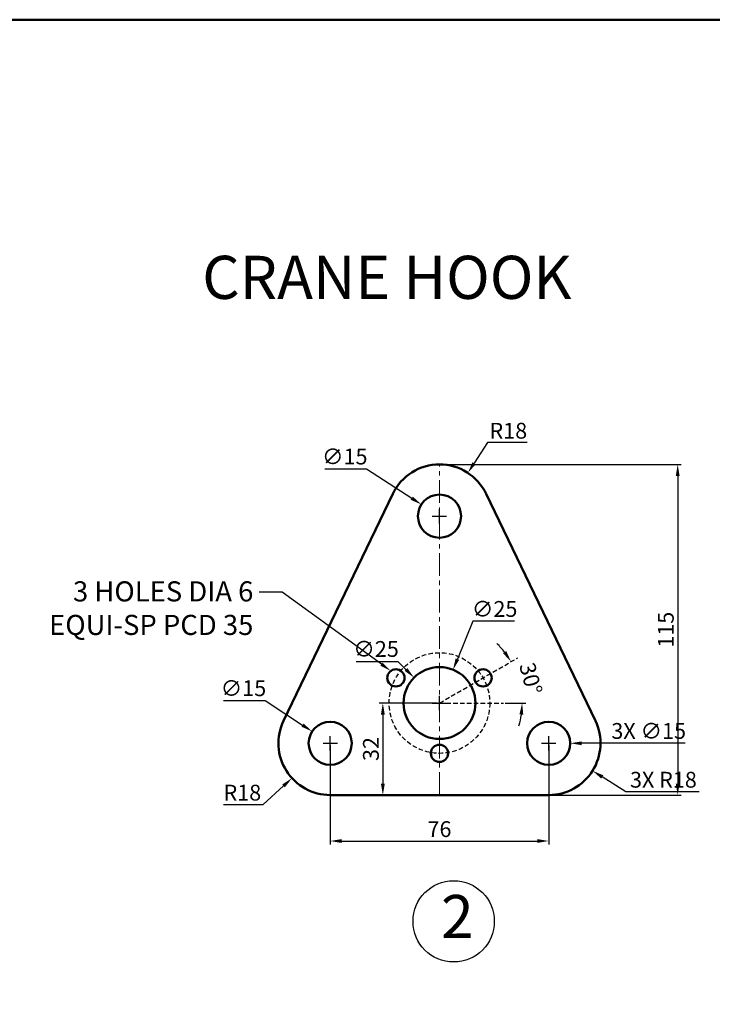
# Model space of a CAD drawing. Units: millimetres. Extents: x -3 to 930, y -425 to 322.
# Tile 4 of 5: x 288 to 529, y -21 to 322. Entities that reach past the tile are written whole.
import ezdxf
from ezdxf import colors
from ezdxf.entities.mleader import LeaderData, LeaderLine
from ezdxf.math import Vec2, Vec3

# ---------------------------------------------------------------- set-up
doc = ezdxf.new("R2010")
doc.units = ezdxf.units.MM
doc.header["$LTSCALE"] = 0.5
doc.linetypes.add('CENTER', pattern=[50.8, 31.75, -6.35, 6.35, -6.35])
doc.linetypes.add('HIDDEN', pattern=[9.525, 6.35, -3.175])
for name, color, linetype, lineweight in [('M-ANNO-SYMB', 3, 'Continuous', 25), ('M-CNTR', 1, 'CENTER', 18), ('M-DIMS', 2, 'Continuous', 25), ('M-HIDN', 4, 'HIDDEN', 25), ('M-OUTL', 7, 'Continuous', 50), ('M-TEXT', 3, 'Continuous', 25)]:
    doc.layers.add(name, color=color, linetype=linetype, lineweight=lineweight)
doc.styles.get("Standard").update_dxf_attribs({"font": 'arial.ttf'})
doc.dimstyles.new('ISO-25', dxfattribs={"dimtxt": 5.5, "dimasz": 4, "dimexe": 1.25, "dimexo": 0.625, "dimtad": 1, "dimtoh": 1, "dimdec": 0, "dimtxsty": 'Standard', "dimcen": 2.5, "dimadec": 0, "dimazin": 0, "dimtfac": 1, "dimtdec": 0, "dimtofl": 0, "dimtmove": 0, "dimatfit": 3, "dimfxl": 1, "dimarcsym": 0})

# ---------------------------------------------------------------- blocks, each defined once
blk = doc.blocks.new('*D19')
at = {"layer": 'Defpoints', "color": 0, "ltscale": 0.5, "transparency": 16777216}
for p in [(396.31, 69.97), (472.31, 69.97), (472.31, 35.98)]:
    blk.add_point(p, dxfattribs=at)
at = {"layer": 'M-DIMS', "color": 0, "lineweight": -2, "ltscale": 0.5, "transparency": 16777216}
for p, q in [((396.31, 69.35), (396.31, 34.73)), ((472.31, 69.35), (472.31, 34.73)), ((400.31, 35.98), (468.31, 35.98))]:
    blk.add_line(p, q, dxfattribs=at)
at = {"layer": 'M-DIMS', "color": 0, "ltscale": 0.5, "transparency": 16777216}
for points in [[(400.31, 36.65), (400.31, 35.31), (396.31, 35.98)], [(468.31, 36.65), (468.31, 35.31), (472.31, 35.98)]]:
    blk.add_solid(points, dxfattribs=at)
at = {"layer": 'M-DIMS', "color": 0, "ltscale": 0.5, "transparency": 16777216, "insert": (434.31, 39.41), "char_height": 5.5, "attachment_point": 5}
blk.add_mtext('76', dxfattribs=at)
blk = doc.blocks.new('*D20')
at = {"layer": 'Defpoints', "color": 0, "ltscale": 0.5, "transparency": 16777216}
for p in [(434.31, 166.97), (434.31, 51.97), (517.16, 51.97)]:
    blk.add_point(p, dxfattribs=at)
at = {"layer": 'M-DIMS', "color": 0, "lineweight": -2, "ltscale": 0.5, "transparency": 16777216}
for p, q in [((434.93, 166.97), (518.41, 166.97)), ((517.16, 162.97), (517.16, 55.97)), ((434.93, 51.97), (518.41, 51.97))]:
    blk.add_line(p, q, dxfattribs=at)
at = {"layer": 'M-DIMS', "color": 0, "ltscale": 0.5, "transparency": 16777216}
for points in [[(516.49, 162.97), (517.83, 162.97), (517.16, 166.97)], [(516.49, 55.97), (517.83, 55.97), (517.16, 51.97)]]:
    blk.add_solid(points, dxfattribs=at)
at = {"layer": 'M-DIMS', "color": 0, "ltscale": 0.5, "transparency": 16777216, "insert": (513.73, 109.47), "char_height": 5.5, "attachment_point": 5, "rotation": 90}
blk.add_mtext('115', dxfattribs=at)
blk = doc.blocks.new('*D21')
at = {"layer": 'Defpoints', "color": 0, "ltscale": 0.5, "transparency": 16777216}
for p in [(396.31, 69.97), (383.02, 57.84)]:
    blk.add_point(p, dxfattribs=at)
at = {"layer": 'M-DIMS', "color": 0, "lineweight": -2, "ltscale": 0.5, "transparency": 16777216}
for p, q in [((396.31, 67.47), (396.31, 72.47)), ((393.81, 69.97), (398.81, 69.97)), ((372.96, 48.65), (380.06, 55.14)), ((359.19, 48.65), (372.96, 48.65))]:
    blk.add_line(p, q, dxfattribs=at)
at = {"layer": 'M-DIMS', "color": 0, "ltscale": 0.5, "transparency": 16777216}
blk.add_solid([(379.62, 55.63), (380.51, 54.65), (383.02, 57.84)], dxfattribs=at)
at = {"layer": 'M-DIMS', "color": 0, "ltscale": 0.5, "transparency": 16777216, "insert": (365.76, 52.09), "char_height": 5.5, "attachment_point": 5}
blk.add_mtext('R18', dxfattribs=at)
blk = doc.blocks.new('*D22')
at = {"layer": 'Defpoints', "color": 0, "ltscale": 0.5, "transparency": 16777216}
for p in [(444.17, 164.03), (434.31, 148.97)]:
    blk.add_point(p, dxfattribs=at)
at = {"layer": 'M-DIMS', "color": 0, "lineweight": -2, "ltscale": 0.5, "transparency": 16777216}
for p, q in [((451.06, 174.55), (446.36, 167.38)), ((464.83, 174.55), (451.06, 174.55)), ((434.31, 146.47), (434.31, 151.47)), ((431.81, 148.97), (436.81, 148.97))]:
    blk.add_line(p, q, dxfattribs=at)
at = {"layer": 'M-DIMS', "color": 0, "ltscale": 0.5, "transparency": 16777216}
blk.add_solid([(445.8, 167.74), (446.92, 167.01), (444.17, 164.03)], dxfattribs=at)
at = {"layer": 'M-DIMS', "color": 0, "ltscale": 0.5, "transparency": 16777216, "insert": (458.26, 177.98), "char_height": 5.5, "attachment_point": 5}
blk.add_mtext('R18', dxfattribs=at)
blk = doc.blocks.new('*D23')
at = {"layer": 'Defpoints', "color": 0, "ltscale": 0.5, "transparency": 16777216}
for p in [(428.02, 153.05), (440.6, 144.89)]:
    blk.add_point(p, dxfattribs=at)
at = {"layer": 'M-DIMS', "color": 0, "lineweight": -2, "ltscale": 0.5, "transparency": 16777216}
for p, q in [((394.42, 165.41), (408.95, 165.41)), ((408.95, 165.41), (424.66, 155.23)), ((434.31, 146.47), (434.31, 151.47)), ((431.81, 148.97), (436.81, 148.97))]:
    blk.add_line(p, q, dxfattribs=at)
at = {"layer": 'M-DIMS', "color": 0, "ltscale": 0.5, "transparency": 16777216}
blk.add_solid([(425.02, 155.79), (424.3, 154.67), (428.02, 153.05)], dxfattribs=at)
at = {"layer": 'M-DIMS', "color": 0, "ltscale": 0.5, "transparency": 16777216, "insert": (401.37, 169), "char_height": 5.5, "attachment_point": 5}
blk.add_mtext('∅15', dxfattribs=at)
blk = doc.blocks.new('*D24')
at = {"layer": 'Defpoints', "color": 0, "ltscale": 0.5, "transparency": 16777216}
for p in [(390.04, 74.09), (402.58, 65.86)]:
    blk.add_point(p, dxfattribs=at)
at = {"layer": 'M-DIMS', "color": 0, "lineweight": -2, "ltscale": 0.5, "transparency": 16777216}
for p, q in [((359.18, 84.82), (373.7, 84.82)), ((373.7, 84.82), (386.7, 76.29)), ((396.31, 67.47), (396.31, 72.47)), ((393.81, 69.97), (398.81, 69.97))]:
    blk.add_line(p, q, dxfattribs=at)
at = {"layer": 'M-DIMS', "color": 0, "ltscale": 0.5, "transparency": 16777216}
blk.add_solid([(387.06, 76.84), (386.33, 75.73), (390.04, 74.09)], dxfattribs=at)
at = {"layer": 'M-DIMS', "color": 0, "ltscale": 0.5, "transparency": 16777216, "insert": (366.13, 88.41), "char_height": 5.5, "attachment_point": 5}
blk.add_mtext('∅15', dxfattribs=at)
blk = doc.blocks.new('*D25')
at = {"layer": 'Defpoints', "color": 0, "ltscale": 0.5, "transparency": 16777216}
for p in [(439.03, 95.55), (429.59, 72.4)]:
    blk.add_point(p, dxfattribs=at)
at = {"layer": 'M-DIMS', "color": 0, "lineweight": -2, "ltscale": 0.5, "transparency": 16777216}
for p, q in [((445.92, 112.41), (440.55, 99.25)), ((460.45, 112.41), (445.92, 112.41)), ((434.31, 81.47), (434.31, 86.47)), ((431.81, 83.97), (436.81, 83.97))]:
    blk.add_line(p, q, dxfattribs=at)
at = {"layer": 'M-DIMS', "color": 0, "ltscale": 0.5, "transparency": 16777216}
blk.add_solid([(439.93, 99.5), (441.16, 99), (439.03, 95.55)], dxfattribs=at)
at = {"layer": 'M-DIMS', "color": 0, "ltscale": 0.5, "transparency": 16777216, "insert": (453.49, 115.99), "char_height": 5.5, "attachment_point": 5}
blk.add_mtext('∅25', dxfattribs=at)
blk = doc.blocks.new('*D26')
at = {"layer": 'Defpoints', "color": 0, "ltscale": 0.5, "transparency": 16777216}
for p in [(461.61, 99.74), (462.63, 88.97), (434.31, 83.97), (434.31, 83.97), (456.56, 83.97)]:
    blk.add_point(p, dxfattribs=at)
at = {"layer": 'M-DIMS', "color": 0, "lineweight": -2, "ltscale": 0.5, "transparency": 16777216}
blk.add_line((457.19, 83.97), (464.32, 83.97), dxfattribs=at)
for start, end in [(37.9764, 45.9529), (344.0471, 352.0236)]:
    blk.add_arc((434.31, 83.97), 28.76, start, end, dxfattribs=at)
at = {"layer": 'M-DIMS', "color": 0, "ltscale": 0.5, "transparency": 16777216}
for points in [[(457.53, 102.04), (456.42, 101.3), (459.21, 98.35)], [(462.12, 80.03), (463.45, 79.94), (463.07, 83.97)]]:
    blk.add_solid(points, dxfattribs=at)
at = {"layer": 'M-DIMS', "color": 0, "ltscale": 0.5, "transparency": 16777216, "insert": (465.4, 92.3), "char_height": 5.5, "attachment_point": 5, "rotation": 285}
blk.add_mtext('30°', dxfattribs=at)
blk = doc.blocks.new('*D27')
at = {"layer": 'Defpoints', "color": 0, "ltscale": 0.5, "transparency": 16777216}
for p in [(434.31, 83.97), (414.62, 51.97), (434.31, 51.97)]:
    blk.add_point(p, dxfattribs=at)
at = {"layer": 'M-DIMS', "color": 0, "lineweight": -2, "ltscale": 0.5, "transparency": 16777216}
for p, q in [((433.68, 83.97), (413.37, 83.97)), ((414.62, 79.97), (414.62, 55.97)), ((433.68, 51.97), (413.37, 51.97))]:
    blk.add_line(p, q, dxfattribs=at)
at = {"layer": 'M-DIMS', "color": 0, "ltscale": 0.5, "transparency": 16777216}
for points in [[(413.95, 79.97), (415.29, 79.97), (414.62, 83.97)], [(413.95, 55.97), (415.29, 55.97), (414.62, 51.97)]]:
    blk.add_solid(points, dxfattribs=at)
at = {"layer": 'M-DIMS', "color": 0, "ltscale": 0.5, "transparency": 16777216, "insert": (411.18, 67.97), "char_height": 5.5, "attachment_point": 5, "rotation": 90}
blk.add_mtext('32', dxfattribs=at)
blk = doc.blocks.new('BALLOON')
at = {"ltscale": 0.5}
blk.add_circle((198.15, 8.03), 14.13, dxfattribs=at)
blk = doc.blocks.new('*D92')
at = {"layer": 'Defpoints', "color": 0, "ltscale": 0.5, "transparency": 16777216}
for p in [(472.31, 69.97), (487.55, 60.39)]:
    blk.add_point(p, dxfattribs=at)
at = {"layer": 'M-DIMS', "color": 0, "lineweight": -2, "ltscale": 0.5, "transparency": 16777216}
for p, q in [((472.31, 67.47), (472.31, 72.47)), ((469.81, 69.97), (474.81, 69.97)), ((499.08, 53.14), (490.94, 58.26)), ((524.67, 53.14), (499.08, 53.14))]:
    blk.add_line(p, q, dxfattribs=at)
at = {"layer": 'M-DIMS', "color": 0, "ltscale": 0.5, "transparency": 16777216}
blk.add_solid([(491.29, 58.83), (490.58, 57.7), (487.55, 60.39)], dxfattribs=at)
at = {"layer": 'M-DIMS', "color": 0, "ltscale": 0.5, "transparency": 16777216, "insert": (512.19, 56.58), "char_height": 5.5, "attachment_point": 5}
blk.add_mtext('3X R18', dxfattribs=at)
blk = doc.blocks.new('*D93')
at = {"layer": 'Defpoints', "color": 0, "ltscale": 0.5, "transparency": 16777216}
for p in [(464.81, 69.98), (479.81, 69.97)]:
    blk.add_point(p, dxfattribs=at)
at = {"layer": 'M-DIMS', "color": 0, "lineweight": -2, "ltscale": 0.5, "transparency": 16777216}
for p, q in [((472.31, 67.47), (472.31, 72.47)), ((469.81, 69.97), (474.81, 69.97)), ((493.73, 69.96), (483.81, 69.97)), ((519.78, 69.96), (493.73, 69.96))]:
    blk.add_line(p, q, dxfattribs=at)
at = {"layer": 'M-DIMS', "color": 0, "ltscale": 0.5, "transparency": 16777216}
blk.add_solid([(483.81, 70.63), (483.81, 69.3), (479.81, 69.97)], dxfattribs=at)
at = {"layer": 'M-DIMS', "color": 0, "ltscale": 0.5, "transparency": 16777216, "insert": (507.07, 73.55), "char_height": 5.5, "attachment_point": 5}
blk.add_mtext('3X ∅15', dxfattribs=at)
blk = doc.blocks.new('*D94')
at = {"layer": 'Defpoints', "color": 0, "ltscale": 0.5, "transparency": 16777216}
for p in [(425.48, 92.82), (443.14, 75.13)]:
    blk.add_point(p, dxfattribs=at)
at = {"layer": 'M-DIMS', "color": 0, "lineweight": -2, "ltscale": 0.5, "transparency": 16777216}
for p, q in [((405.3, 98.48), (419.83, 98.48)), ((419.83, 98.48), (422.65, 95.65)), ((434.31, 81.47), (434.31, 86.47)), ((431.81, 83.97), (436.81, 83.97))]:
    blk.add_line(p, q, dxfattribs=at)
at = {"layer": 'M-DIMS', "color": 0, "ltscale": 0.5, "transparency": 16777216}
blk.add_solid([(423.13, 96.12), (422.18, 95.18), (425.48, 92.82)], dxfattribs=at)
at = {"layer": 'M-DIMS', "color": 0, "ltscale": 0.5, "transparency": 16777216, "insert": (412.25, 102.07), "char_height": 5.5, "attachment_point": 5}
blk.add_mtext('∅25', dxfattribs=at)

msp = doc.modelspace()

# ---------------------------------------------------------------- linework, layer by layer
at = {"layer": 'M-CNTR', "ltscale": 0.5}
msp.add_line((434.3099, 51.9733), (434.3099, 166.9733), dxfattribs=at)
at = {"layer": 'M-HIDN', "ltscale": 0.5}
for q in [(461.6109, 99.7356), (456.5633, 83.9733)]:
    msp.add_line((434.3099, 83.9733), q, dxfattribs=at)
msp.add_circle((434.3099, 83.9733), 17.5, dxfattribs=at)
at = {"layer": 'M-OUTL', "ltscale": 0.5}
for p, q in [((418.0889, 156.7759), (380.0889, 77.7759)), ((450.5309, 156.7759), (488.5309, 77.7759)), ((396.3099, 51.9733), (472.3099, 51.9733))]:
    msp.add_line(p, q, dxfattribs=at)
msp.add_lwpolyline([(-2.6134, 321.6785), (929.6113, 321.6785), (929.6113, -424.8872), (-2.6134, -424.8872)], close=True, dxfattribs=at)
for centre, radius in [((434.3099, 148.9733), 7.5), ((434.3099, 83.9733), 12.5), ((419.1545, 92.7233), 3), ((449.4654, 92.7233), 3), ((396.3099, 69.9733), 7.5), ((472.3099, 69.9733), 7.5), ((434.3099, 66.4733), 3)]:
    msp.add_circle(centre, radius, dxfattribs=at)
for centre, start, end in [((434.3099, 148.9733), 25.688143, 154.311857), ((396.3099, 69.9733), 154.311857, 270), ((472.3099, 69.9733), 270, 25.688143)]:
    msp.add_arc(centre, 18, start, end, dxfattribs=at)

# ---------------------------------------------------------------- block references
at = {"layer": 'M-ANNO-SYMB'}
msp.add_blockref('BALLOON', (241.1008, 0), dxfattribs=at)

# ---------------------------------------------------------------- texts
at = {"layer": 'M-TEXT', "ltscale": 0.5, "char_height": 15, "attachment_point": 1}
for s, width, insert in [('CRANE HOOK', 189.287448, (351.7987, 239.5512)), ('2', 15, (434.8526, 17.2084))]:
    msp.add_mtext_dynamic_manual_height_columns(s, width=width, gutter_width=12.5, heights=[0], dxfattribs=dict(at, insert=insert))

# ---------------------------------------------------------------- dimensions: what is measured, and where the dimension line sits
at = {"layer": 'M-DIMS', "ltscale": 0.5}
dim = msp.add_radius_dim(center=(434.3099, 148.9733), mpoint=(444.1699, 164.0326), dimstyle='ISO-25', override={"dimclrd": 0, "dimclre": 0, "dimclrt": 0}, dxfattribs=at)
dim.commit()
dim.dimension.update_dxf_attribs({"geometry": '*D22', "text_midpoint": (458.2571, 174.549), "dimtype": 164})
for p1, p2, override, picture, middle in [((440.6035, 144.894), (428.0164, 153.0527), {"dimclrd": 0, "dimclre": 0, "dimclrt": 0}, '*D23', (401.3735, 165.4108)), ((429.5856, 72.4005), (439.0342, 95.5462), {"dimclrd": 0, "dimclre": 0, "dimclrt": 0}, '*D25', (453.4933, 112.405)), ((443.1404, 75.1261), (425.4795, 92.8206), {"dimdec": 0, "dimlfac": 1, "dimrnd": 0, "dimzin": 0, "dimdsep": 46, "dimlunit": 2}, '*D94', (412.2511, 98.4828)), ((402.5787, 65.8561), (390.0411, 74.0906), {"dimclrd": 0, "dimclre": 0, "dimclrt": 0}, '*D24', (366.1273, 84.8206))]:
    dim = msp.add_diameter_dim_2p(p1=p1, p2=p2, dimstyle='ISO-25', override=override, dxfattribs=at)
    dim.commit()
    dim.dimension.update_dxf_attribs({"geometry": picture, "text_midpoint": middle, "dimtype": 163})
for base, p1, picture, middle in [((517.1601, 51.9733), (434.3099, 166.9733), '*D20', (513.7269, 109.4733)), ((414.6186, 51.9733), (434.3099, 83.9733), '*D27', (411.1836, 67.9733))]:
    dim = msp.add_linear_dim(base=base, p1=p1, p2=(434.3099, 51.9733), angle=90, dimstyle='ISO-25', override={"dimclrd": 0, "dimclre": 0, "dimclrt": 0}, dxfattribs=at)
    dim.commit()
    dim.dimension.update_dxf_attribs({"geometry": picture, "text_midpoint": middle})
dim = msp.add_angular_dim_2l(base=(462.6288, 88.9667), line1=((434.3099, 83.9733), (456.5633, 83.9733)), line2=((434.3099, 83.9733), (461.6109, 99.7356)), dimstyle='ISO-25', override={"dimclrd": 0, "dimclre": 0, "dimclrt": 0}, dxfattribs=at)
dim.commit()
dim.dimension.update_dxf_attribs({"geometry": '*D26', "text_midpoint": (465.4038, 92.3049)})
dim = msp.add_diameter_dim_2p(p1=(464.8099, 69.9767), p2=(479.8099, 69.97), text='3X <>', dimstyle='ISO-25', override={"dimdec": 0, "dimlfac": 1, "dimrnd": 0, "dimzin": 0, "dimdsep": 46, "dimlunit": 2}, dxfattribs=at)
dim.commit()
dim.dimension.update_dxf_attribs({"geometry": '*D93', "text_midpoint": (493.7339, 69.9638), "dimtype": 163})
dim = msp.add_radius_dim(center=(396.3099, 69.9733), mpoint=(383.0185, 57.8351), dimstyle='ISO-25', override={"dimclrd": 0, "dimclre": 0, "dimclrt": 0}, dxfattribs=at)
dim.commit()
dim.dimension.update_dxf_attribs({"geometry": '*D21', "text_midpoint": (365.7623, 52.0861)})
dim = msp.add_radius_dim(center=(472.3099, 69.9733), mpoint=(487.5487, 60.3932), text='3X <>', dimstyle='ISO-25', override={"dimdec": 0, "dimlfac": 1, "dimrnd": 0, "dimzin": 0, "dimdsep": 46, "dimlunit": 2}, dxfattribs=at)
dim.commit()
dim.dimension.update_dxf_attribs({"geometry": '*D92', "text_midpoint": (512.1882, 56.5792)})
dim = msp.add_linear_dim(base=(472.3099, 35.9783), p1=(396.3099, 69.9733), p2=(472.3099, 69.9733), dimstyle='ISO-25', override={"dimclrd": 0, "dimclre": 0, "dimclrt": 0}, dxfattribs=at)
dim.commit()
dim.dimension.update_dxf_attribs({"geometry": '*D19', "text_midpoint": (434.3099, 39.4115)})

# ---------------------------------------------------------------- leaders
ml = msp.add_multileader_mtext('Standard', dxfattribs=at)
ml.set_content('3 HOLES DIA 6\\PEQUI-SP PCD 35', color=256)
ml.set_leader_properties()
ml.build(insert=Vec2(0, 0))
ctx = ml.context
ctx.base_point, ctx.char_height, ctx.plane_origin = Vec3(291.5867, 122.5424), 7, Vec3(417.3699, 95.1348)
ctx.text_align_type = 2
notes = []
notes.append((ctx, [(0, (1, 1, 0), (379.5887, 122.5424), (-1, 0), 8, [(0, [(417.3699, 95.1348)], 0, [])])]))
ctx.mtext.insert, ctx.mtext.alignment, ctx.mtext.flow_direction = Vec3(369.5887, 126.3146), 3, 5
for ctx, leaders in notes:
    for number, flags, end, landing, length, lines in leaders:
        leader = LeaderData()
        leader.index, (leader.has_last_leader_line, leader.has_dogleg_vector, leader.attachment_direction) = number, flags
        leader.last_leader_point, leader.dogleg_vector, leader.dogleg_length = Vec3(end), Vec3(landing), length
        for number, points, colour, breaks in lines:
            line = LeaderLine()
            line.index, line.vertices, line.color, line.breaks = number, Vec3.list(points), colors.encode_raw_color(colour), breaks
            leader.lines.append(line)
        ctx.leaders.append(leader)

doc.saveas('drawing.dxf')
